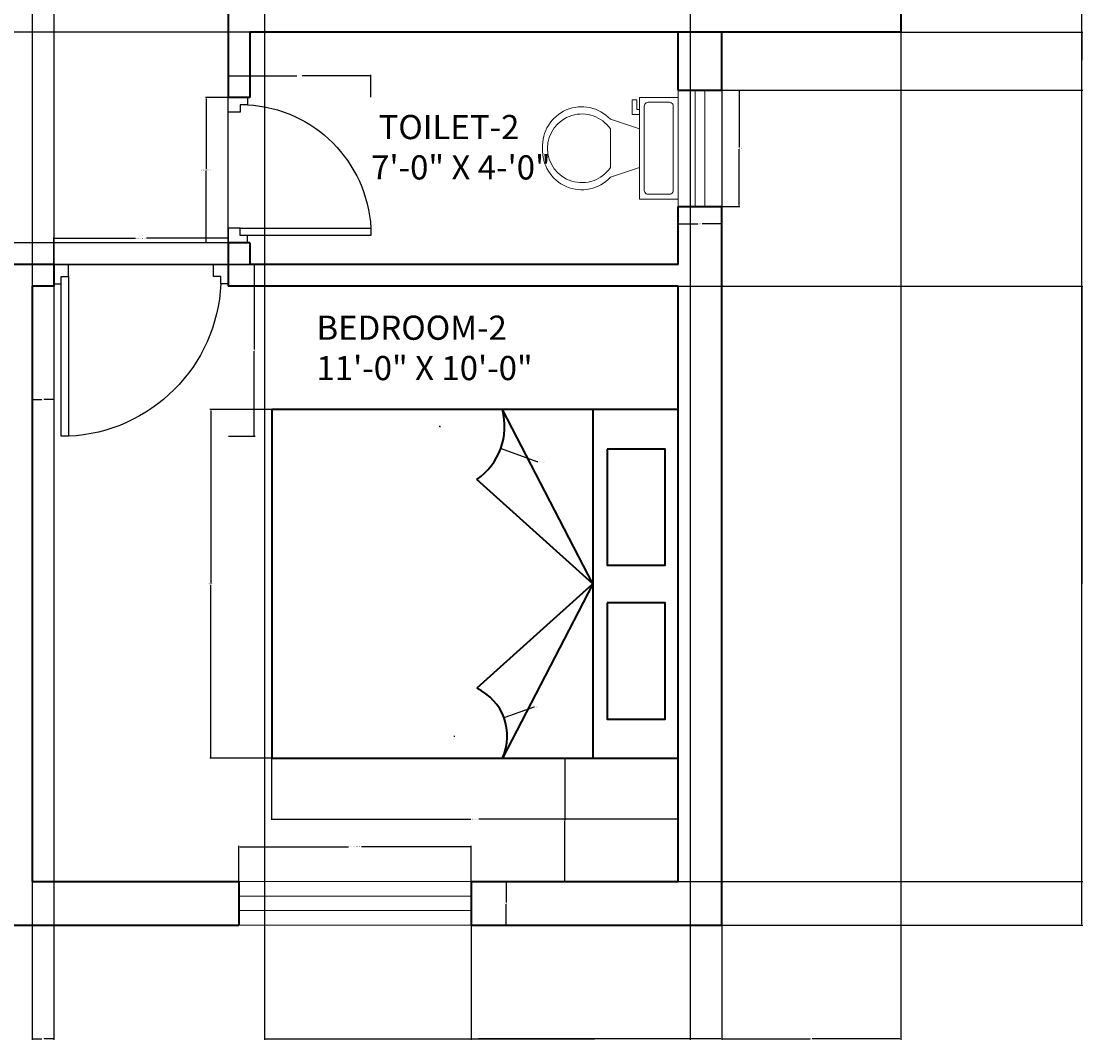
# Model space of a CAD drawing. Units: inches. Extents: x 324 to 662, y 102 to 605.
# Tile 2 of 4: x 443 to 662, y 102 to 313. Entities that reach past the tile are written whole.
import ezdxf

# ---------------------------------------------------------------- set-up
doc = ezdxf.new("R2010")
doc.units = ezdxf.units.IN
for name, color, linetype, lineweight in [('A-ANNO-DIMS', 2, 'Continuous', 18), ('A-AREA-IDEN', 7, 'Continuous', 25), ('A-FLOR-FIXT', 8, 'Continuous', 18), ('door', 82, 'Continuous', 25), ('furniture', 8, 'Continuous', 18), ('ventilator', 20, 'Continuous', 18), ('wall', 7, 'Continuous', 35), ('window', 50, 'Continuous', 18)]:
    doc.layers.add(name, color=color, linetype=linetype, lineweight=lineweight)
doc.styles.get("Standard").update_dxf_attribs({"font": 'arial.ttf'})
doc.dimstyles.get("Standard").update_dxf_attribs({"dimtxt": 0.18, "dimasz": 0.18, "dimexe": 0.18, "dimexo": 0.0625, "dimgap": 0.09, "dimtad": 0, "dimtih": 1, "dimtoh": 1, "dimdec": 4, "dimzin": 0, "dimdsep": 46, "dimtxsty": 'Standard', "dimcen": 0.09, "dimadec": 0, "dimazin": 0, "dimtfac": 1, "dimtdec": 4, "dimtofl": 0, "dimtmove": 0, "dimatfit": 3, "dimfxl": 1, "dimtolj": 1, "dimtzin": 0, "dimarcsym": 0})

# ---------------------------------------------------------------- blocks, each defined once
blk = doc.blocks.new('d2')
at = {"layer": 'door'}
blk.add_line((825.6, 261.67), (855.6, 261.67), dxfattribs=at)
blk.add_lwpolyline([(827.1, 264.17), (828.6, 264.17), (828.6, 291.17), (827.1, 291.17)], close=True, dxfattribs=at)
for points in [[(828.6, 261.67), (825.6, 261.67), (825.6, 265.67), (827.1, 265.67), (827.1, 264.17), (828.6, 264.17), (828.6, 261.67)], [(852.6, 261.67), (855.6, 261.67), (855.6, 265.67), (854.1, 265.67), (854.1, 264.17), (852.6, 264.17), (852.6, 261.67)]]:
    blk.add_lwpolyline(points, dxfattribs=at)
blk.add_arc((827.1, 264.17), 27.04, 3.1798, 86.8202, dxfattribs=at)
blk = doc.blocks.new('w1')
at = {"layer": 'window'}
for p, q in [((719.66, 290.3), (719.66, 242.3)), ((722.66, 290.3), (722.66, 242.3))]:
    blk.add_line(p, q, dxfattribs=at)
blk.add_lwpolyline([(716.66, 242.3), (725.66, 242.3), (725.66, 290.3), (716.66, 290.3)], close=True, dxfattribs=at)
blk = doc.blocks.new('v')
at = {"layer": 'ventilator'}
for p, q in [((1044.91, 377.37), (1044.91, 353.37)), ((1046.91, 377.37), (1046.91, 353.37))]:
    blk.add_line(p, q, dxfattribs=at)
blk.add_lwpolyline([(1041.41, 377.37), (1050.41, 377.37), (1050.41, 353.37), (1041.41, 353.37)], close=True, dxfattribs=at)
blk = doc.blocks.new('d1')
at = {"layer": 'door'}
blk.add_line((825.6, 316.36), (861.6, 316.36), dxfattribs=at)
blk.add_lwpolyline([(827.1, 318.86), (828.6, 318.86), (828.6, 351.86), (827.1, 351.86)], close=True, dxfattribs=at)
for points in [[(828.6, 316.36), (825.6, 316.36), (825.6, 320.36), (827.1, 320.36), (827.1, 318.86), (828.6, 318.86), (828.6, 316.36)], [(858.6, 316.36), (861.6, 316.36), (861.6, 320.36), (860.1, 320.36), (860.1, 318.86), (858.6, 318.86), (858.6, 316.36)]]:
    blk.add_lwpolyline(points, dxfattribs=at)
blk.add_arc((827.1, 318.86), 33.03, 2.6026, 87.3974, dxfattribs=at)
blk = doc.blocks.new('BED')
at = {"layer": 'wall'}
for p, q in [((215.01, 591.25), (287.01, 591.25)), ((251.01, 591.25), (215.01, 572.55)), ((251.01, 591.25), (229.44, 567.26)), ((251.01, 591.25), (287.01, 572.55)), ((251.01, 591.25), (272.58, 567.26))]:
    blk.add_line(p, q, dxfattribs=at)
for points in [[(215.01, 524.86), (287.01, 524.86), (287.01, 608.86), (215.01, 608.86)], [(223.15, 594.21), (247.15, 594.21), (247.15, 606.21), (223.15, 606.21)], [(254.93, 594.21), (278.93, 594.21), (278.93, 606.21), (254.93, 606.21)]]:
    blk.add_lwpolyline(points, close=True, dxfattribs=at)
for centre, radius, start, end in [((218.46, 559.65), 13.35, 34.7262, 104.9976), ((282.46, 562.63), 10.92, 65.3787, 154.8976)]:
    blk.add_arc(centre, radius, start, end, dxfattribs=at)
blk = doc.blocks.new('*U8')
for p, q in [((9.5, -6), (9.5, -2)), ((-10, -8.5), (-8, -8.5)), ((-10, -9.5), (-10, -8.5)), ((-8, -8.5), (-8, -8)), ((-7, -8), (-7, -9.5)), ((-4, -8), (-6, -14)), ((4, -8), (6, -14)), ((-7, -9.5), (-10, -9.5)), ((4, -14), (-4, -14))]:
    blk.add_line(p, q)
blk.add_lwpolyline([(10.5, -8), (10.5, 0), (-10.5, 0), (-10.5, -8)], close=True)
for points in [[(-9.5, -2), (-9.5, -6)], [(8.5, -1), (-8.5, -1)], [(-8.5, -7), (8.5, -7)]]:
    blk.add_lwpolyline(points)
for centre, radius, start, end in [((-8.625, -1.875), 0.8839, 81.8699, 188.1301), ((8.625, -1.875), 0.8839, 351.8699, 98.1301), ((-8.625, -6.125), 0.8839, 171.869898, 278.1301), ((8.625, -6.125), 0.8839, 261.8699, 8.1301), ((-0.4772, -19.9188), 8.0953, 133.01722, 273.38), ((0.0374, -19.8731), 7.127, 124.50543, 269.7), ((-0.0373, -19.8731), 7.127, 270.3, 55.4946), ((0.4773, -19.9188), 8.0953, 266.62, 46.9828)]:
    blk.add_arc(centre, radius, start, end)
blk = doc.blocks.new('*D10')
at = {"layer": 'A-ANNO-DIMS', "color": 0, "lineweight": -2, "transparency": 16777216}
for p, q in [((449.83, 262.42), (449.83, 267.94)), ((450.01, 267.76), (466.7, 267.76)), ((485.65, 267.76), (468.96, 267.76)), ((485.83, 262.42), (485.83, 267.94))]:
    blk.add_line(p, q, dxfattribs=at)
at = {"layer": 'A-ANNO-DIMS', "color": 0, "transparency": 16777216}
for points in [[(450.01, 267.79), (450.01, 267.73), (449.83, 267.76)], [(485.65, 267.79), (485.65, 267.73), (485.83, 267.76)]]:
    blk.add_solid(points, dxfattribs=at)
at = {"layer": 'Defpoints', "color": 0, "transparency": 16777216}
for p in [(485.83, 267.76), (449.83, 262.36), (485.83, 262.36)]:
    blk.add_point(p, dxfattribs=at)
at = {"layer": 'A-ANNO-DIMS', "color": 0, "transparency": 16777216, "insert": (467.83, 267.76), "char_height": 0.18, "attachment_point": 5}
blk.add_mtext('\\A1;DOOR D1 36 TYP.', dxfattribs=at)
blk = doc.blocks.new('*D11')
at = {"layer": 'A-ANNO-DIMS', "color": 0, "lineweight": -2, "transparency": 16777216}
for p, q in [((485.89, 262.36), (491.41, 262.36)), ((491.23, 262.18), (491.23, 244.79)), ((491.23, 227.04), (491.23, 244.43)), ((485.89, 226.86), (491.41, 226.86))]:
    blk.add_line(p, q, dxfattribs=at)
at = {"layer": 'A-ANNO-DIMS', "color": 0, "transparency": 16777216}
for points in [[(491.2, 262.18), (491.26, 262.18), (491.23, 262.36)], [(491.2, 227.04), (491.26, 227.04), (491.23, 226.86)]]:
    blk.add_solid(points, dxfattribs=at)
at = {"layer": 'Defpoints', "color": 0, "transparency": 16777216}
for p in [(485.83, 262.36), (485.83, 226.86), (491.23, 226.86)]:
    blk.add_point(p, dxfattribs=at)
at = {"layer": 'A-ANNO-DIMS', "color": 0, "transparency": 16777216, "insert": (491.23, 244.61), "char_height": 0.18, "attachment_point": 5}
blk.add_mtext('\\A1;36 TYP.', dxfattribs=at)
blk = doc.blocks.new('*D12')
at = {"layer": 'A-ANNO-DIMS', "color": 0, "lineweight": -2, "transparency": 16777216}
for p, q in [((485.77, 296.86), (481.15, 296.86)), ((481.33, 296.68), (481.33, 282.04)), ((481.33, 267.04), (481.33, 281.68)), ((485.77, 266.86), (481.15, 266.86))]:
    blk.add_line(p, q, dxfattribs=at)
at = {"layer": 'A-ANNO-DIMS', "color": 0, "transparency": 16777216}
for points in [[(481.3, 296.68), (481.36, 296.68), (481.33, 296.86)], [(481.3, 267.04), (481.36, 267.04), (481.33, 266.86)]]:
    blk.add_solid(points, dxfattribs=at)
at = {"layer": 'Defpoints', "color": 0, "transparency": 16777216}
for p in [(481.33, 296.86), (485.83, 296.86), (485.83, 266.86)]:
    blk.add_point(p, dxfattribs=at)
at = {"layer": 'A-ANNO-DIMS', "color": 0, "transparency": 16777216, "insert": (481.33, 281.86), "char_height": 0.18, "attachment_point": 5}
blk.add_mtext('\\A1;DOOR D2 30 TYP.', dxfattribs=at)
blk = doc.blocks.new('*D13')
at = {"layer": 'A-ANNO-DIMS', "color": 0, "lineweight": -2, "transparency": 16777216}
for p, q in [((485.83, 296.92), (485.83, 301.54)), ((486.01, 301.36), (500.05, 301.36)), ((515.15, 301.36), (501.11, 301.36)), ((515.33, 296.92), (515.33, 301.54))]:
    blk.add_line(p, q, dxfattribs=at)
at = {"layer": 'A-ANNO-DIMS', "color": 0, "transparency": 16777216}
for points in [[(486.01, 301.39), (486.01, 301.33), (485.83, 301.36)], [(515.15, 301.39), (515.15, 301.33), (515.33, 301.36)]]:
    blk.add_solid(points, dxfattribs=at)
at = {"layer": 'Defpoints', "color": 0, "transparency": 16777216}
for p in [(515.33, 301.36), (485.83, 296.86), (515.33, 296.86)]:
    blk.add_point(p, dxfattribs=at)
at = {"layer": 'A-ANNO-DIMS', "color": 0, "transparency": 16777216, "insert": (500.58, 301.36), "char_height": 0.18, "attachment_point": 5}
blk.add_mtext('\\A1;30 TYP.', dxfattribs=at)
blk = doc.blocks.new('*D14')
at = {"layer": 'A-ANNO-DIMS', "color": 0, "lineweight": -2, "transparency": 16777216}
for p, q in [((488.08, 134.92), (488.08, 142.24)), ((488.26, 142.06), (510.74, 142.06)), ((535.9, 142.06), (513.42, 142.06)), ((536.08, 134.92), (536.08, 142.24))]:
    blk.add_line(p, q, dxfattribs=at)
at = {"layer": 'A-ANNO-DIMS', "color": 0, "transparency": 16777216}
for points in [[(488.26, 142.09), (488.26, 142.03), (488.08, 142.06)], [(535.9, 142.09), (535.9, 142.03), (536.08, 142.06)]]:
    blk.add_solid(points, dxfattribs=at)
at = {"layer": 'Defpoints', "color": 0, "transparency": 16777216}
for p in [(488.08, 142.06), (488.08, 134.86), (536.08, 134.86)]:
    blk.add_point(p, dxfattribs=at)
at = {"layer": 'A-ANNO-DIMS', "color": 0, "transparency": 16777216, "insert": (512.08, 142.06), "char_height": 0.18, "attachment_point": 5}
blk.add_mtext('\\A1;WINDOW W1 48 TYP.', dxfattribs=at)
blk = doc.blocks.new('*D15')
at = {"layer": 'A-ANNO-DIMS', "color": 0, "lineweight": -2, "transparency": 16777216}
for p, q in [((536.14, 134.86), (543.46, 134.86)), ((543.28, 134.68), (543.28, 130.54)), ((543.28, 126.04), (543.28, 130.18)), ((536.14, 125.86), (543.46, 125.86))]:
    blk.add_line(p, q, dxfattribs=at)
at = {"layer": 'A-ANNO-DIMS', "color": 0, "transparency": 16777216}
for points in [[(543.25, 134.68), (543.31, 134.68), (543.28, 134.86)], [(543.25, 126.04), (543.31, 126.04), (543.28, 125.86)]]:
    blk.add_solid(points, dxfattribs=at)
at = {"layer": 'Defpoints', "color": 0, "transparency": 16777216}
for p in [(536.08, 134.86), (543.28, 134.86), (536.08, 125.86)]:
    blk.add_point(p, dxfattribs=at)
at = {"layer": 'A-ANNO-DIMS', "color": 0, "transparency": 16777216, "insert": (543.28, 130.36), "char_height": 0.18, "attachment_point": 5}
blk.add_mtext('\\A1;9 TYP.', dxfattribs=at)
blk = doc.blocks.new('*D18')
at = {"layer": 'A-ANNO-DIMS', "color": 0, "lineweight": -2, "transparency": 16777216}
for p, q in [((587.89, 298.36), (591.61, 298.36)), ((591.43, 298.18), (591.43, 286.54)), ((591.43, 274.54), (591.43, 286.18)), ((587.89, 274.36), (591.61, 274.36))]:
    blk.add_line(p, q, dxfattribs=at)
at = {"layer": 'A-ANNO-DIMS', "color": 0, "transparency": 16777216}
for points in [[(591.4, 298.18), (591.46, 298.18), (591.43, 298.36)], [(591.4, 274.54), (591.46, 274.54), (591.43, 274.36)]]:
    blk.add_solid(points, dxfattribs=at)
at = {"layer": 'Defpoints', "color": 0, "transparency": 16777216}
for p in [(587.83, 298.36), (591.43, 298.36), (587.83, 274.36)]:
    blk.add_point(p, dxfattribs=at)
at = {"layer": 'A-ANNO-DIMS', "color": 0, "transparency": 16777216, "insert": (591.43, 286.36), "char_height": 0.18, "attachment_point": 5}
blk.add_mtext('\\A1;VENT 24 TYP.', dxfattribs=at)
blk = doc.blocks.new('*D19')
at = {"layer": 'A-ANNO-DIMS', "color": 0, "lineweight": -2, "transparency": 16777216}
for p, q in [((578.83, 274.3), (578.83, 270.58)), ((587.83, 274.3), (587.83, 270.58)), ((579.01, 270.76), (582.87, 270.76)), ((587.65, 270.76), (583.79, 270.76))]:
    blk.add_line(p, q, dxfattribs=at)
at = {"layer": 'A-ANNO-DIMS', "color": 0, "transparency": 16777216}
for points in [[(579.01, 270.79), (579.01, 270.73), (578.83, 270.76)], [(587.65, 270.79), (587.65, 270.73), (587.83, 270.76)]]:
    blk.add_solid(points, dxfattribs=at)
at = {"layer": 'Defpoints', "color": 0, "transparency": 16777216}
for p in [(578.83, 274.36), (587.83, 274.36), (587.83, 270.76)]:
    blk.add_point(p, dxfattribs=at)
at = {"layer": 'A-ANNO-DIMS', "color": 0, "transparency": 16777216, "insert": (583.33, 270.76), "char_height": 0.18, "attachment_point": 5}
blk.add_mtext('\\A1;9 TYP.', dxfattribs=at)
blk = doc.blocks.new('*D20')
at = {"layer": 'A-ANNO-DIMS', "color": 0, "lineweight": -2, "transparency": 16777216}
for p, q in [((494.83, 160.3), (494.83, 147.58)), ((578.83, 160.3), (578.83, 147.58)), ((495.01, 147.76), (536.01, 147.76)), ((578.65, 147.76), (537.65, 147.76))]:
    blk.add_line(p, q, dxfattribs=at)
at = {"layer": 'A-ANNO-DIMS', "color": 0, "transparency": 16777216}
for points in [[(495.01, 147.79), (495.01, 147.73), (494.83, 147.76)], [(578.65, 147.79), (578.65, 147.73), (578.83, 147.76)]]:
    blk.add_solid(points, dxfattribs=at)
at = {"layer": 'Defpoints', "color": 0, "transparency": 16777216}
for p in [(494.83, 160.36), (578.83, 160.36), (578.83, 147.76)]:
    blk.add_point(p, dxfattribs=at)
at = {"layer": 'A-ANNO-DIMS', "color": 0, "transparency": 16777216, "insert": (536.83, 147.76), "char_height": 0.18, "attachment_point": 5}
blk.add_mtext('\\A1;BED 84 TYP.', dxfattribs=at)
blk = doc.blocks.new('*D21')
at = {"layer": 'A-ANNO-DIMS', "color": 0, "lineweight": -2, "transparency": 16777216}
for p, q in [((494.77, 232.36), (482.05, 232.36)), ((482.23, 232.18), (482.23, 196.54)), ((482.23, 160.54), (482.23, 196.18)), ((494.77, 160.36), (482.05, 160.36))]:
    blk.add_line(p, q, dxfattribs=at)
at = {"layer": 'A-ANNO-DIMS', "color": 0, "transparency": 16777216}
for points in [[(482.2, 232.18), (482.26, 232.18), (482.23, 232.36)], [(482.2, 160.54), (482.26, 160.54), (482.23, 160.36)]]:
    blk.add_solid(points, dxfattribs=at)
at = {"layer": 'Defpoints', "color": 0, "transparency": 16777216}
for p in [(494.83, 232.36), (482.23, 160.36), (494.83, 160.36)]:
    blk.add_point(p, dxfattribs=at)
at = {"layer": 'A-ANNO-DIMS', "color": 0, "transparency": 16777216, "insert": (482.23, 196.36), "char_height": 0.18, "attachment_point": 5}
blk.add_mtext('\\A1;72 TYP.', dxfattribs=at)
blk = doc.blocks.new('*D25')
at = {"layer": 'A-ANNO-DIMS', "color": 0, "lineweight": -2, "transparency": 16777216}
for p, q in [((587.89, 581.86), (662.43, 581.86)), ((662.25, 581.68), (662.25, 354.04)), ((662.25, 126.04), (662.25, 353.68)), ((587.89, 125.86), (662.43, 125.86))]:
    blk.add_line(p, q, dxfattribs=at)
at = {"layer": 'A-ANNO-DIMS', "color": 0, "transparency": 16777216}
for points in [[(662.22, 581.68), (662.28, 581.68), (662.25, 581.86)], [(662.22, 126.04), (662.28, 126.04), (662.25, 125.86)]]:
    blk.add_solid(points, dxfattribs=at)
at = {"layer": 'Defpoints', "color": 0, "transparency": 16777216}
for p in [(587.83, 581.86), (587.83, 125.86), (662.25, 125.86)]:
    blk.add_point(p, dxfattribs=at)
at = {"layer": 'A-ANNO-DIMS', "color": 0, "transparency": 16777216, "insert": (662.25, 353.86), "char_height": 0.18, "attachment_point": 5}
blk.add_mtext('\\A1;456', dxfattribs=at)
blk = doc.blocks.new('*D26')
at = {"layer": 'A-ANNO-DIMS', "color": 0, "lineweight": -2, "transparency": 16777216}
for p, q in [((587.83, 310.3), (587.83, 102.17)), ((624.83, 310.3), (624.83, 102.17)), ((588.01, 102.35), (606.11, 102.35)), ((624.65, 102.35), (606.55, 102.35))]:
    blk.add_line(p, q, dxfattribs=at)
at = {"layer": 'A-ANNO-DIMS', "color": 0, "transparency": 16777216}
for points in [[(588.01, 102.38), (588.01, 102.32), (587.83, 102.35)], [(624.65, 102.38), (624.65, 102.32), (624.83, 102.35)]]:
    blk.add_solid(points, dxfattribs=at)
at = {"layer": 'Defpoints', "color": 0, "transparency": 16777216}
for p in [(587.83, 310.36), (624.83, 310.36), (624.83, 102.35)]:
    blk.add_point(p, dxfattribs=at)
at = {"layer": 'A-ANNO-DIMS', "color": 0, "transparency": 16777216, "insert": (606.33, 102.35), "char_height": 0.18, "attachment_point": 5}
blk.add_mtext('\\A1;37', dxfattribs=at)
blk = doc.blocks.new('*D34')
at = {"layer": 'A-ANNO-DIMS', "color": 0, "lineweight": -2, "transparency": 16777216}
for p, q in [((490.27, 403.36), (324.24, 403.36)), ((324.42, 403.18), (324.42, 357.04)), ((324.42, 310.54), (324.42, 356.68)), ((490.27, 310.36), (324.24, 310.36))]:
    blk.add_line(p, q, dxfattribs=at)
at = {"layer": 'A-ANNO-DIMS', "color": 0, "transparency": 16777216}
for points in [[(324.39, 403.18), (324.45, 403.18), (324.42, 403.36)], [(324.39, 310.54), (324.45, 310.54), (324.42, 310.36)]]:
    blk.add_solid(points, dxfattribs=at)
at = {"layer": 'Defpoints', "color": 0, "transparency": 16777216}
for p in [(490.33, 403.36), (324.42, 310.36), (490.33, 310.36)]:
    blk.add_point(p, dxfattribs=at)
at = {"layer": 'A-ANNO-DIMS', "color": 0, "transparency": 16777216, "insert": (324.42, 356.86), "char_height": 0.18, "attachment_point": 5}
blk.add_mtext('\\A1;93', dxfattribs=at)
blk = doc.blocks.new('*D37')
at = {"layer": 'A-ANNO-DIMS', "color": 0, "lineweight": -2, "transparency": 16777216}
for p, q in [((587.89, 310.36), (662.43, 310.36)), ((662.25, 310.18), (662.25, 304.54)), ((662.25, 298.54), (662.25, 304.18)), ((587.89, 298.36), (662.43, 298.36))]:
    blk.add_line(p, q, dxfattribs=at)
at = {"layer": 'A-ANNO-DIMS', "color": 0, "transparency": 16777216}
for points in [[(662.22, 310.18), (662.28, 310.18), (662.25, 310.36)], [(662.22, 298.54), (662.28, 298.54), (662.25, 298.36)]]:
    blk.add_solid(points, dxfattribs=at)
at = {"layer": 'Defpoints', "color": 0, "transparency": 16777216}
for p in [(587.83, 310.36), (587.83, 298.36), (662.25, 298.36)]:
    blk.add_point(p, dxfattribs=at)
at = {"layer": 'A-ANNO-DIMS', "color": 0, "transparency": 16777216, "insert": (662.25, 304.36), "char_height": 0.18, "attachment_point": 5}
blk.add_mtext('\\A1;12', dxfattribs=at)
blk = doc.blocks.new('*D38')
at = {"layer": 'A-ANNO-DIMS', "color": 0, "lineweight": -2, "transparency": 16777216}
for p, q in [((536.08, 125.8), (536.08, 102.17)), ((587.83, 125.8), (587.83, 102.17)), ((536.26, 102.35), (561.56, 102.35)), ((587.65, 102.35), (562.35, 102.35))]:
    blk.add_line(p, q, dxfattribs=at)
at = {"layer": 'A-ANNO-DIMS', "color": 0, "transparency": 16777216}
for points in [[(536.26, 102.38), (536.26, 102.32), (536.08, 102.35)], [(587.65, 102.38), (587.65, 102.32), (587.83, 102.35)]]:
    blk.add_solid(points, dxfattribs=at)
at = {"layer": 'Defpoints', "color": 0, "transparency": 16777216}
for p in [(536.08, 125.86), (587.83, 125.86), (536.08, 102.35)]:
    blk.add_point(p, dxfattribs=at)
at = {"layer": 'A-ANNO-DIMS', "color": 0, "transparency": 16777216, "insert": (561.96, 102.35), "char_height": 0.18, "attachment_point": 5}
blk.add_mtext('\\A1;51.75', dxfattribs=at)
blk = doc.blocks.new('*D44')
at = {"layer": 'A-ANNO-DIMS', "color": 0, "lineweight": -2, "transparency": 16777216}
for p, q in [((493.33, 314.8), (493.33, 102.17)), ((581.33, 314.8), (581.33, 102.17)), ((493.51, 102.35), (537.11, 102.35)), ((581.15, 102.35), (537.55, 102.35))]:
    blk.add_line(p, q, dxfattribs=at)
at = {"layer": 'A-ANNO-DIMS', "color": 0, "transparency": 16777216}
for points in [[(493.51, 102.38), (493.51, 102.32), (493.33, 102.35)], [(581.15, 102.38), (581.15, 102.32), (581.33, 102.35)]]:
    blk.add_solid(points, dxfattribs=at)
at = {"layer": 'Defpoints', "color": 0, "transparency": 16777216}
for p in [(493.33, 314.86), (581.33, 314.86), (581.33, 102.35)]:
    blk.add_point(p, dxfattribs=at)
at = {"layer": 'A-ANNO-DIMS', "color": 0, "transparency": 16777216, "insert": (537.33, 102.35), "char_height": 0.18, "attachment_point": 5}
blk.add_mtext('\\A1;88', dxfattribs=at)
blk = doc.blocks.new('*D52')
at = {"layer": 'A-ANNO-DIMS', "color": 0, "lineweight": -2, "transparency": 16777216}
for p, q in [((445.33, 455.8), (445.33, 102.17)), ((449.83, 451.3), (449.83, 102.17)), ((445.51, 102.35), (447.32, 102.35)), ((449.65, 102.35), (447.84, 102.35))]:
    blk.add_line(p, q, dxfattribs=at)
at = {"layer": 'A-ANNO-DIMS', "color": 0, "transparency": 16777216}
for points in [[(445.51, 102.38), (445.51, 102.32), (445.33, 102.35)], [(449.65, 102.38), (449.65, 102.32), (449.83, 102.35)]]:
    blk.add_solid(points, dxfattribs=at)
at = {"layer": 'Defpoints', "color": 0, "transparency": 16777216}
for p in [(445.33, 455.86), (449.83, 451.36), (449.83, 102.35)]:
    blk.add_point(p, dxfattribs=at)
at = {"layer": 'A-ANNO-DIMS', "color": 0, "transparency": 16777216, "insert": (447.58, 102.35), "char_height": 0.18, "attachment_point": 5}
blk.add_mtext('\\A1;4.5', dxfattribs=at)
blk = doc.blocks.new('*D54')
at = {"layer": 'A-ANNO-DIMS', "color": 0, "lineweight": -2, "transparency": 16777216}
for p, q in [((485.77, 266.86), (324.24, 266.86)), ((324.42, 266.68), (324.42, 264.79)), ((324.42, 262.54), (324.42, 264.43)), ((490.27, 262.36), (324.24, 262.36))]:
    blk.add_line(p, q, dxfattribs=at)
at = {"layer": 'A-ANNO-DIMS', "color": 0, "transparency": 16777216}
for points in [[(324.39, 266.68), (324.45, 266.68), (324.42, 266.86)], [(324.39, 262.54), (324.45, 262.54), (324.42, 262.36)]]:
    blk.add_solid(points, dxfattribs=at)
at = {"layer": 'Defpoints', "color": 0, "transparency": 16777216}
for p in [(485.83, 266.86), (324.42, 262.36), (490.33, 262.36)]:
    blk.add_point(p, dxfattribs=at)
at = {"layer": 'A-ANNO-DIMS', "color": 0, "transparency": 16777216, "insert": (324.42, 264.61), "char_height": 0.18, "attachment_point": 5}
blk.add_mtext('\\A1;4.5', dxfattribs=at)
blk = doc.blocks.new('*D55')
at = {"layer": 'A-ANNO-DIMS', "color": 0, "lineweight": -2, "transparency": 16777216}
for p, q in [((578.77, 160.36), (555.24, 160.36)), ((555.42, 160.18), (555.42, 147.79)), ((555.42, 135.04), (555.42, 147.43)), ((578.77, 134.86), (555.24, 134.86))]:
    blk.add_line(p, q, dxfattribs=at)
at = {"layer": 'A-ANNO-DIMS', "color": 0, "transparency": 16777216}
for points in [[(555.39, 160.18), (555.45, 160.18), (555.42, 160.36)], [(555.39, 135.04), (555.45, 135.04), (555.42, 134.86)]]:
    blk.add_solid(points, dxfattribs=at)
at = {"layer": 'Defpoints', "color": 0, "transparency": 16777216}
for p in [(555.42, 160.36), (578.83, 160.36), (578.83, 134.86)]:
    blk.add_point(p, dxfattribs=at)
at = {"layer": 'A-ANNO-DIMS', "color": 0, "transparency": 16777216, "insert": (555.42, 147.61), "char_height": 0.18, "attachment_point": 5}
blk.add_mtext('\\A1;25.5', dxfattribs=at)
blk = doc.blocks.new('*D61')
at = {"layer": 'A-ANNO-DIMS', "color": 0, "lineweight": -2, "transparency": 16777216}
for p, q in [((578.89, 257.86), (662.43, 257.86)), ((662.25, 257.68), (662.25, 196.54)), ((662.25, 135.04), (662.25, 196.18)), ((578.89, 134.86), (662.43, 134.86))]:
    blk.add_line(p, q, dxfattribs=at)
at = {"layer": 'A-ANNO-DIMS', "color": 0, "transparency": 16777216}
for points in [[(662.22, 257.68), (662.28, 257.68), (662.25, 257.86)], [(662.22, 135.04), (662.28, 135.04), (662.25, 134.86)]]:
    blk.add_solid(points, dxfattribs=at)
at = {"layer": 'Defpoints', "color": 0, "transparency": 16777216}
for p in [(578.83, 257.86), (662.25, 257.86), (578.83, 134.86)]:
    blk.add_point(p, dxfattribs=at)
at = {"layer": 'A-ANNO-DIMS', "color": 0, "transparency": 16777216, "insert": (662.25, 196.36), "char_height": 0.18, "attachment_point": 5}
blk.add_mtext('\\A1;123', dxfattribs=at)
blk = doc.blocks.new('*D63')
at = {"layer": 'A-ANNO-DIMS', "color": 0, "lineweight": -2, "transparency": 16777216}
for p, q in [((445.33, 257.8), (445.33, 234.26)), ((449.83, 257.8), (449.83, 234.26)), ((445.51, 234.44), (447.32, 234.44)), ((449.65, 234.44), (447.84, 234.44))]:
    blk.add_line(p, q, dxfattribs=at)
at = {"layer": 'A-ANNO-DIMS', "color": 0, "transparency": 16777216}
for points in [[(445.51, 234.47), (445.51, 234.41), (445.33, 234.44)], [(449.65, 234.47), (449.65, 234.41), (449.83, 234.44)]]:
    blk.add_solid(points, dxfattribs=at)
at = {"layer": 'Defpoints', "color": 0, "transparency": 16777216}
for p in [(445.33, 257.86), (449.83, 257.86), (445.33, 234.44)]:
    blk.add_point(p, dxfattribs=at)
at = {"layer": 'A-ANNO-DIMS', "color": 0, "transparency": 16777216, "insert": (447.58, 234.44), "char_height": 0.18, "attachment_point": 5}
blk.add_mtext('\\A1;4.5', dxfattribs=at)
blk = doc.blocks.new('*D71')
at = {"layer": 'A-ANNO-DIMS', "color": 0, "lineweight": -2, "transparency": 16777216}
for p, q in [((529.53, 228.9), (529.71, 228.9)), ((529.62, 228.81), (529.62, 228.99)), ((549.69, 221.55), (542.33, 224.24)), ((549.87, 221.55), (549.69, 221.55))]:
    blk.add_line(p, q, dxfattribs=at)
at = {"layer": 'A-ANNO-DIMS', "color": 0, "transparency": 16777216}
blk.add_solid([(542.34, 224.27), (542.32, 224.22), (542.16, 224.31)], dxfattribs=at)
at = {"layer": 'Defpoints', "color": 0, "transparency": 16777216}
for p in [(529.62, 228.9), (542.16, 224.31)]:
    blk.add_point(p, dxfattribs=at)
at = {"layer": 'A-ANNO-DIMS', "color": 0, "transparency": 16777216, "insert": (550.61, 221.55), "char_height": 0.18, "attachment_point": 5}
blk.add_mtext('\\A1;2X R13.354', dxfattribs=at)
blk = doc.blocks.new('*D72')
at = {"layer": 'A-ANNO-DIMS', "color": 0, "lineweight": -2, "transparency": 16777216}
for p, q in [((549, 170.92), (543.02, 168.73)), ((549.18, 170.92), (549, 170.92)), ((532.51, 164.91), (532.69, 164.91)), ((532.6, 164.82), (532.6, 165))]:
    blk.add_line(p, q, dxfattribs=at)
at = {"layer": 'A-ANNO-DIMS', "color": 0, "transparency": 16777216}
blk.add_solid([(543.01, 168.75), (543.03, 168.7), (542.85, 168.66)], dxfattribs=at)
at = {"layer": 'Defpoints', "color": 0, "transparency": 16777216}
for p in [(542.85, 168.66), (532.6, 164.91)]:
    blk.add_point(p, dxfattribs=at)
at = {"layer": 'A-ANNO-DIMS', "color": 0, "transparency": 16777216, "insert": (549.92, 170.92), "char_height": 0.18, "attachment_point": 5}
blk.add_mtext('\\A1;2X R10.915', dxfattribs=at)

msp = doc.modelspace()

# ---------------------------------------------------------------- linework, layer by layer
at = {"layer": 'wall'}
for p, q in [((624.8304, 326.8598), (624.8304, 310.3598)), ((485.8304, 314.8598), (485.8304, 296.8598)), ((624.8304, 310.3598), (490.3304, 310.3598)), ((490.3304, 310.3598), (490.3304, 296.8598)), ((578.8304, 298.3598), (578.8304, 310.3598)), ((587.8304, 298.3598), (587.8304, 310.3598)), ((578.8304, 298.3598), (587.8304, 298.3598)), ((490.3304, 296.8598), (485.8304, 296.8598)), ((578.8304, 262.3598), (578.8304, 274.3598)), ((578.8304, 274.3598), (587.8304, 274.3598)), ((587.8304, 125.8598), (587.8304, 274.3598)), ((490.3304, 266.8598), (485.8304, 266.8598)), ((485.8304, 266.8598), (485.8304, 262.3598)), ((490.3304, 266.8598), (490.3304, 262.3598)), ((449.8304, 262.3598), (436.3304, 262.3598)), ((449.8304, 262.3598), (449.8304, 257.8598)), ((485.8304, 262.3598), (485.8304, 257.8598)), ((578.8304, 262.3598), (490.3304, 262.3598)), ((445.3304, 257.8598), (445.3304, 134.8598)), ((449.8304, 257.8598), (445.3304, 257.8598)), ((578.8304, 257.8598), (485.8304, 257.8598)), ((578.8304, 134.8598), (578.8304, 257.8598)), ((445.3304, 134.8598), (488.0804, 134.8598)), ((488.0804, 134.8598), (488.0804, 125.8598)), ((536.0804, 134.8598), (536.0804, 125.8598)), ((536.0804, 134.8598), (578.8304, 134.8598)), ((440.8304, 125.8598), (488.0804, 125.8598)), ((536.0804, 125.8598), (587.8304, 125.8598))]:
    msp.add_line(p, q, dxfattribs=at)

# ---------------------------------------------------------------- block references
at = {"layer": 'A-FLOR-FIXT', "rotation": 270}
msp.add_blockref('*U8', (578.8304, 286.3598), dxfattribs=at)
at = {"layer": 'door', "xscale": -1}
for name, p, rotation in [('d2', (224.1615, -558.7449), 270), ('d1', (-375.7743, 578.7154), 180)]:
    msp.add_blockref(name, p, dxfattribs=dict(at, rotation=rotation))
at = {"layer": 'furniture', "rotation": 270}
msp.add_blockref('BED', (-30.0254, 447.3668), dxfattribs=at)
at = {"layer": 'ventilator'}
msp.add_blockref('v', (-462.5774, -79.0135), dxfattribs=at)
at = {"layer": 'window', "rotation": 90}
msp.add_blockref('w1', (778.385, -590.7975), dxfattribs=at)

# ---------------------------------------------------------------- texts
at = {"layer": 'A-AREA-IDEN', "char_height": 5, "attachment_point": 1}
for s, insert in [(' TOILET-2\\P7\'-0" X 4-\'0"', (515.3898, 293.2477)), ('BEDROOM-2\\P11\'-0" X 10\'-0"', (504.0914, 251.7914))]:
    msp.add_mtext_dynamic_manual_height_columns(s, width=50.156641, gutter_width=12.5, heights=[0], dxfattribs=dict(at, insert=insert))

# ---------------------------------------------------------------- dimensions: what is measured, and where the dimension line sits
at = {"layer": 'A-ANNO-DIMS'}
for base, p1, p2, angle, override, picture, middle in [((662.2454, 125.8598), (587.8304, 581.8598), (587.8304, 125.8598), 90, {"dimdec": 0, "dimlfac": 1, "dimrnd": 0, "dimzin": 0, "dimdsep": 46, "dimlunit": 2}, '*D25', (662.2454, 353.8598)), ((324.4154, 310.3598), (490.3304, 403.3598), (490.3304, 310.3598), 90, {"dimdec": 0, "dimlfac": 1, "dimrnd": 0, "dimzin": 0, "dimdsep": 46, "dimlunit": 2}, '*D34', (324.4154, 356.8598)), ((662.2454, 298.3598), (587.8304, 310.3598), (587.8304, 298.3598), 90, {"dimdec": 0, "dimlfac": 1, "dimrnd": 0, "dimzin": 0, "dimdsep": 46, "dimlunit": 2}, '*D37', (662.2454, 304.3598)), ((324.4154, 262.3598), (485.8304, 266.8598), (490.3304, 262.3598), 90, {"dimdec": 1, "dimlfac": 1, "dimrnd": 0, "dimzin": 0, "dimdsep": 46, "dimlunit": 2}, '*D54', (324.4154, 264.6098)), ((445.3304, 234.4448), (449.8304, 257.8598), (445.3304, 257.8598), 180, {"dimdec": 1, "dimlfac": 1, "dimrnd": 0, "dimzin": 0, "dimdsep": 46, "dimlunit": 2}, '*D63', (447.5804, 234.4448)), ((662.2454, 257.8598), (578.8304, 134.8598), (578.8304, 257.8598), 90, {"dimdec": 0, "dimlfac": 1, "dimrnd": 0, "dimzin": 0, "dimdsep": 46, "dimlunit": 2}, '*D61', (662.2454, 196.3598)), ((555.4154, 160.3598), (578.8304, 134.8598), (578.8304, 160.3598), 90, {"dimdec": 1, "dimlfac": 1, "dimrnd": 0, "dimzin": 0, "dimdsep": 46, "dimlunit": 2}, '*D55', (555.4154, 147.6098))]:
    dim = msp.add_linear_dim(base=base, p1=p1, p2=p2, angle=angle, dimstyle='Standard', override=override, dxfattribs=at)
    dim.commit()
    dim.dimension.update_dxf_attribs({"geometry": picture, "text_midpoint": middle})
for base, p1, p2, override, picture, middle in [((449.8304, 102.3527), (445.3304, 455.8598), (449.8304, 451.3598), {"dimdec": 1, "dimlfac": 1, "dimrnd": 0, "dimzin": 0, "dimdsep": 46, "dimlunit": 2}, '*D52', (447.5804, 102.3527)), ((581.3304, 102.3527), (493.3304, 314.8598), (581.3304, 314.8598), {"dimdec": 0, "dimlfac": 1, "dimrnd": 0, "dimzin": 0, "dimdsep": 46, "dimlunit": 2}, '*D44', (537.3304, 102.3527)), ((624.8304, 102.3527), (587.8304, 310.3598), (624.8304, 310.3598), {"dimdec": 0, "dimlfac": 1, "dimrnd": 0, "dimzin": 0, "dimdsep": 46, "dimlunit": 2}, '*D26', (606.3304, 102.3527)), ((536.0804, 102.3527), (587.8304, 125.8598), (536.0804, 125.8598), {"dimdec": 2, "dimlfac": 1, "dimrnd": 0, "dimzin": 0, "dimdsep": 46, "dimlunit": 2}, '*D38', (561.9554, 102.3527))]:
    dim = msp.add_linear_dim(base=base, p1=p1, p2=p2, dimstyle='Standard', override=override, dxfattribs=at)
    dim.commit()
    dim.dimension.update_dxf_attribs({"geometry": picture, "text_midpoint": middle})
for base, p1, p2, text, picture, middle in [((515.3303851652, 301.3597676446), (485.8303851652, 296.8597676446), (515.3303851652, 296.8597676446), '<> TYP.', '*D13', (500.5803851652, 301.3597676446)), ((587.8304, 270.7598), (578.8304, 274.3598), (587.8304, 274.3598), '<> TYP.', '*D19', (583.3304, 270.7598)), ((485.8304, 267.7598), (449.8304, 262.3598), (485.8304, 262.3598), 'DOOR D1 <> TYP.', '*D10', (467.8304, 267.7598)), ((578.8304, 147.7598), (494.8304, 160.3598), (578.8304, 160.3598), 'BED <> TYP.', '*D20', (536.8304, 147.7598))]:
    dim = msp.add_linear_dim(base=base, p1=p1, p2=p2, text=text, dimstyle='Standard', override={"dimdec": 0, "dimlfac": 1, "dimrnd": 0, "dimzin": 0, "dimdsep": 46, "dimlunit": 2}, dxfattribs=at)
    dim.commit()
    dim.dimension.update_dxf_attribs({"geometry": picture, "text_midpoint": middle})
for base, p1, p2, angle, text, picture, middle in [((591.4304, 298.3598), (587.8304, 274.3598), (587.8304, 298.3598), 90, 'VENT <> TYP.', '*D18', (591.4304, 286.3598)), ((481.3304, 296.8598), (485.8304, 266.8598), (485.8304, 296.8598), 90, 'DOOR D2 <> TYP.', '*D12', (481.3304, 281.8598)), ((491.2303851652, 226.8597676446), (485.8303851652, 262.3597676446), (485.8303851652, 226.8597676446), 270, '<> TYP.', '*D11', (491.2303851652, 244.6097676446)), ((482.2304, 160.3598), (494.8304, 232.3598), (494.8304, 160.3598), 270, '<> TYP.', '*D21', (482.2304, 196.3598)), ((488.0804, 142.0598), (536.0804, 134.8598), (488.0804, 134.8598), 180, 'WINDOW W1 <> TYP.', '*D14', (512.0804, 142.0598)), ((543.2804, 134.8598), (536.0804, 125.8598), (536.0804, 134.8598), 90, '<> TYP.', '*D15', (543.2804, 130.3598))]:
    dim = msp.add_linear_dim(base=base, p1=p1, p2=p2, angle=angle, text=text, dimstyle='Standard', override={"dimdec": 0, "dimlfac": 1, "dimrnd": 0, "dimzin": 0, "dimdsep": 46, "dimlunit": 2}, dxfattribs=at)
    dim.commit()
    dim.dimension.update_dxf_attribs({"geometry": picture, "text_midpoint": middle})
for center, mpoint, picture, middle in [((529.6249, 228.9039), (542.1628, 224.3061), '*D71', (550.6099, 221.5473)), ((532.6018, 164.9072), (542.8496, 168.6649), '*D72', (549.9237, 170.9194))]:
    dim = msp.add_radius_dim(center=center, mpoint=mpoint, text='2X <>', dimstyle='Standard', override={"dimdec": 3, "dimlfac": 1, "dimrnd": 0, "dimzin": 0, "dimdsep": 46, "dimlunit": 2}, dxfattribs=at)
    dim.commit()
    dim.dimension.update_dxf_attribs({"geometry": picture, "text_midpoint": middle, "dimtype": 164})

doc.saveas('drawing.dxf')
